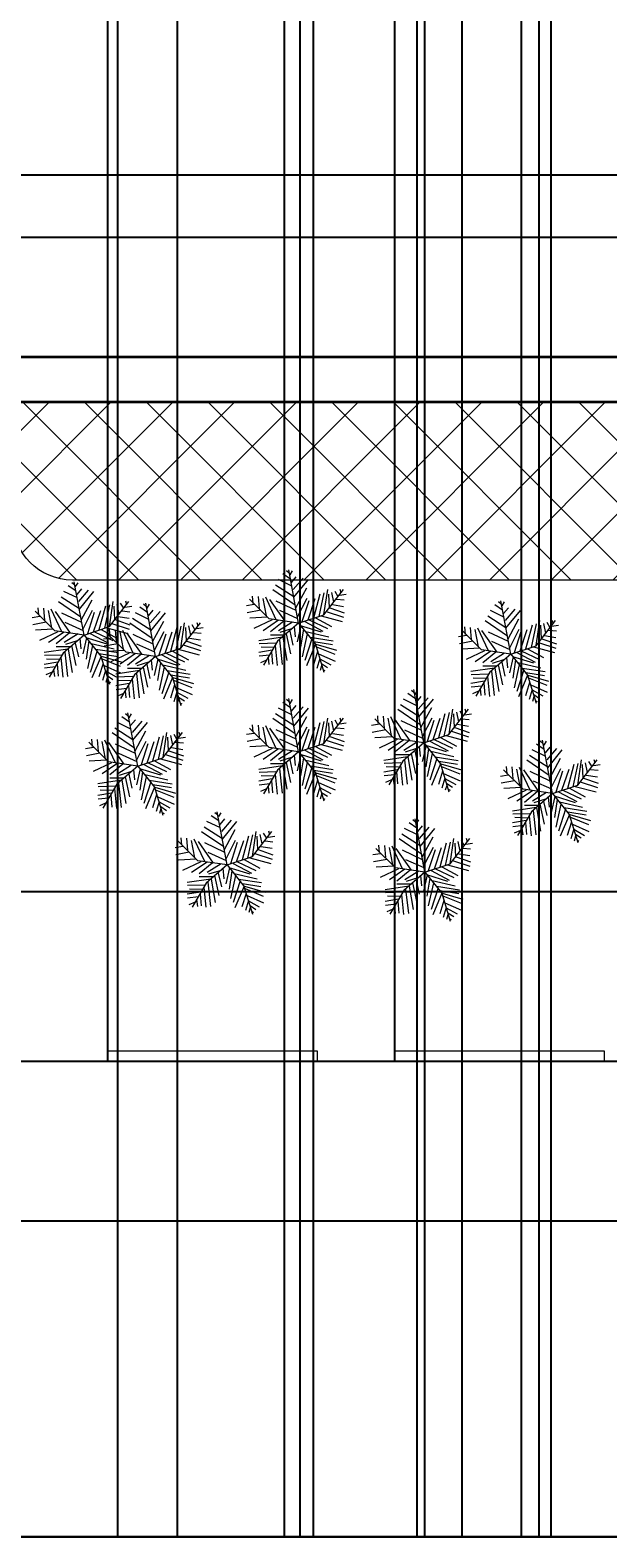
# Model space of a CAD drawing. Units: inches. Extents: x 818 to 1898, y 976 to 2364.
# Tile 16 of 96: x 1434 to 1550, y 976 to 1277. Entities that reach past the tile are written whole.
import ezdxf

# ---------------------------------------------------------------- set-up
doc = ezdxf.new("R2010")
doc.units = ezdxf.units.IN
doc.header["$LTSCALE"] = 5
doc.header["$MEASUREMENT"] = 0
for name, color, linetype, lineweight in [('A-ANNO-DIMS', 2, 'Continuous', 18), ('C-PAVE-PATT', 8, 'Continuous', 9), ('C-PROP', 7, 'Continuous', 35), ('C-ROAD', 8, 'Continuous', 25), ('C-ROAD-MRKG', 7, 'Continuous', 13), ('L-PAVE', 8, 'Continuous', 18)]:
    doc.layers.add(name, color=color, linetype=linetype, lineweight=lineweight)
doc.layers.add('L-PLNT', color=116, linetype='Continuous', lineweight=13, true_color=0x136734)
doc.styles.get("Standard").update_dxf_attribs({"font": 'arial.ttf'})
doc.dimstyles.get("Standard").update_dxf_attribs({"dimtxt": 0.18, "dimasz": 0.18, "dimexe": 0.18, "dimexo": 0.0625, "dimgap": 0.09, "dimtad": 0, "dimtih": 1, "dimtoh": 1, "dimdec": 4, "dimzin": 0, "dimdsep": 46, "dimtxsty": 'Standard', "dimcen": 0.09, "dimadec": 0, "dimazin": 0, "dimtfac": 1, "dimtdec": 4, "dimtofl": 0, "dimtmove": 0, "dimatfit": 3, "dimfxl": 1, "dimtolj": 1, "dimtzin": 0, "dimarcsym": 0})

# ---------------------------------------------------------------- blocks, each defined once
blk = doc.blocks.new('SHRUB-ACCENT')
for p, q in [((9.08, 17.24), (6.37, 18.54)), ((8.8, 18.63), (7.25, 19.67)), ((8.53, 19.84), (7.99, 20.28)), ((10.44, 9.82), (8.47, 20.47)), ((8.74, 19.5), (9.21, 20.28)), ((9.01, 17.93), (9.96, 19.06)), ((9.35, 16.54), (11.31, 18.8)), ((9.48, 14.98), (12.39, 18.54)), ((1.35, 13.77), (1.22, 15.24)), ((2.3, 15.16), (2.51, 12.72)), ((9.75, 13.42), (5.28, 16.46)), ((9.48, 15.07), (5.82, 17.41)), ((9.89, 12.9), (12.06, 16.89)), ((13.48, 10.9), (14.76, 15.68)), ((14.56, 11.16), (15.58, 15.85)), ((15.49, 11.5), (19.41, 16.55)), ((15.51, 11.51), (16.25, 16.54)), ((16.39, 15.59), (16.53, 12.9)), ((17, 15.94), (17.41, 14.03)), ((17.68, 16.2), (18.29, 15.16)), ((18.62, 15.42), (19.98, 15.59)), ((18.69, 16.63), (18.9, 15.94)), ((1.56, 13.51), (0, 13.25)), ((2.84, 12.38), (0.14, 11.86)), ((4.55, 10.66), (0.62, 14.58)), ((3.25, 14.72), (3.93, 11.25)), ((3.79, 15.07), (5.89, 10.55)), ((7.72, 10.21), (4.67, 14.55)), ((5.89, 14.29), (9.89, 12.38)), ((6.57, 12.38), (10.23, 10.73)), ((10.23, 11.07), (12.12, 14.81)), ((11.17, 10.12), (12.53, 14.37)), ((12.33, 10.47), (13.75, 14.72)), ((15.98, 12.12), (19.44, 10.99)), ((16.66, 12.9), (19.57, 11.86)), ((17.2, 13.51), (19.44, 13.16)), ((18.02, 14.63), (19.57, 14.46)), ((4.2, 10.99), (0.68, 10.81)), ((5.15, 10.47), (1.49, 8.73)), ((6.43, 10.38), (3.32, 8.3)), ((10.44, 9.82), (4.55, 10.66)), ((7.45, 10.21), (4.81, 8.04)), ((10.44, 9.82), (6.23, 6.17)), ((9.21, 10.03), (6.43, 8.3)), ((9.55, 9.16), (9.75, 7.08)), ((10.9, 9.25), (10.16, 6.04)), ((10.44, 9.82), (15.49, 11.5)), ((10.44, 9.82), (13.8, 5.61)), ((10.77, 9.34), (14.97, 8.04)), ((11.65, 10.12), (15.31, 8.21)), ((12.53, 10.47), (16.19, 8.73)), ((13.82, 10.9), (17, 9.16)), ((14.97, 11.25), (19.17, 10.12)), ((7.18, 6.99), (2.44, 6.3)), ((6.23, 6.17), (3.43, 1.4)), ((7.59, 7.43), (4.81, 7.43)), ((6.57, 6.39), (7.11, 1.52)), ((9.21, 8.73), (6.7, 7.95)), ((7.25, 6.99), (8.06, 2.31)), ((7.92, 7.69), (8.8, 3.69)), ((8.67, 8.21), (9.28, 5.43)), ((11.38, 8.64), (10.84, 5)), ((12.12, 7.69), (11.11, 3.09)), ((13.07, 6.65), (11.65, 2.31)), ((11.85, 8.12), (16.46, 7.08)), ((12.73, 6.99), (17.34, 6.3)), ((13.48, 6.13), (17.2, 5.52)), ((5.15, 4.39), (2.44, 3.95)), ((5.89, 5.78), (2.51, 5.69)), ((4.67, 3.43), (2.51, 3.17)), ((5.42, 4.91), (2.91, 5)), ((5.01, 4.04), (5.21, 1.61)), ((5.76, 5.34), (6.16, 1.35)), ((13.82, 5.6), (11.99, 1.26)), ((14.22, 4.13), (13.41, 1.44)), ((13.8, 5.61), (15.49, 0)), ((13.88, 5.6), (18.02, 4.39)), ((14.02, 5.08), (17.68, 3.61)), ((14.43, 3.69), (17.74, 2.22)), ((4, 2.39), (2.78, 1.87)), ((4.33, 2.91), (4.47, 1.52)), ((14.7, 2.74), (14.09, 0.74)), ((14.7, 2.65), (16.86, 1.44)), ((15.04, 1.26), (14.76, 0.31)), ((15.04, 1.7), (16.19, 0.92)), ((15.44, 0.48), (15.71, 0.31))]:
    blk.add_line(p, q)
blk = doc.blocks.new('LANE-STRIPE')
at = {"ltscale": 5}
for p, q in [((0, 2), (42, 2)), ((0, 2), (0, 0)), ((0, 0), (42, 0)), ((42, 2), (42, 0))]:
    blk.add_line(p, q, dxfattribs=at)
blk = doc.blocks.new('*D56')
at = {"layer": 'A-ANNO-DIMS', "color": 0, "lineweight": -2, "ltscale": 5, "transparency": 16777216}
for p, q in [((885.95, 1167.31), (885.95, 975.66)), ((1828.91, 1167.31), (1828.91, 975.66)), ((886.13, 975.84), (1357.14, 975.84)), ((1828.73, 975.84), (1357.72, 975.84))]:
    blk.add_line(p, q, dxfattribs=at)
at = {"layer": 'A-ANNO-DIMS', "color": 0, "ltscale": 5, "transparency": 16777216}
for points in [[(886.13, 975.87), (886.13, 975.81), (885.95, 975.84)], [(1828.73, 975.87), (1828.73, 975.81), (1828.91, 975.84)]]:
    blk.add_solid(points, dxfattribs=at)
at = {"layer": 'Defpoints', "color": 0, "ltscale": 5, "transparency": 16777216}
for p in [(885.95, 1167.37), (1828.91, 1167.37), (1828.91, 975.84)]:
    blk.add_point(p, dxfattribs=at)
at = {"layer": 'A-ANNO-DIMS', "color": 0, "ltscale": 5, "transparency": 16777216, "insert": (1357.43, 975.84), "char_height": 0.18, "attachment_point": 5}
blk.add_mtext('\\A1;943', dxfattribs=at)
blk = doc.blocks.new('*D58')
at = {"layer": 'A-ANNO-DIMS', "color": 0, "lineweight": -2, "ltscale": 5, "transparency": 16777216}
for p, q in [((881.51, 1159.31), (881.51, 975.66)), ((1834.44, 1145.13), (1834.44, 975.66)), ((881.69, 975.84), (1357.68, 975.84)), ((1834.26, 975.84), (1358.26, 975.84))]:
    blk.add_line(p, q, dxfattribs=at)
at = {"layer": 'A-ANNO-DIMS', "color": 0, "ltscale": 5, "transparency": 16777216}
for points in [[(881.69, 975.87), (881.69, 975.81), (881.51, 975.84)], [(1834.26, 975.87), (1834.26, 975.81), (1834.44, 975.84)]]:
    blk.add_solid(points, dxfattribs=at)
at = {"layer": 'Defpoints', "color": 0, "ltscale": 5, "transparency": 16777216}
for p in [(881.51, 1159.38), (1834.44, 1145.19), (1834.44, 975.84)]:
    blk.add_point(p, dxfattribs=at)
at = {"layer": 'A-ANNO-DIMS', "color": 0, "ltscale": 5, "transparency": 16777216, "insert": (1357.97, 975.84), "char_height": 0.18, "attachment_point": 5}
blk.add_mtext('\\A1;953', dxfattribs=at)
blk = doc.blocks.new('*D65')
at = {"layer": 'A-ANNO-DIMS', "color": 0, "lineweight": -2, "ltscale": 5, "transparency": 16777216}
for p, q in [((1430.73, 1346.02), (1430.73, 975.66)), ((1714.73, 1346.02), (1714.73, 975.66)), ((1430.91, 975.84), (1572.44, 975.84)), ((1714.55, 975.84), (1573.02, 975.84))]:
    blk.add_line(p, q, dxfattribs=at)
at = {"layer": 'A-ANNO-DIMS', "color": 0, "ltscale": 5, "transparency": 16777216}
for points in [[(1430.91, 975.87), (1430.91, 975.81), (1430.73, 975.84)], [(1714.55, 975.87), (1714.55, 975.81), (1714.73, 975.84)]]:
    blk.add_solid(points, dxfattribs=at)
at = {"layer": 'Defpoints', "color": 0, "ltscale": 5, "transparency": 16777216}
for p in [(1430.73, 1346.08), (1714.73, 1346.08), (1714.73, 975.84)]:
    blk.add_point(p, dxfattribs=at)
at = {"layer": 'A-ANNO-DIMS', "color": 0, "ltscale": 5, "transparency": 16777216, "insert": (1572.73, 975.84), "char_height": 0.18, "attachment_point": 5}
blk.add_mtext('\\A1;284', dxfattribs=at)
blk = doc.blocks.new('*D89')
at = {"layer": 'A-ANNO-DIMS', "color": 0, "lineweight": -2, "ltscale": 5, "transparency": 16777216}
for p, q in [((905.01, 1071.06), (1897.92, 1071.06)), ((1897.74, 1070.88), (1897.74, 1055.28)), ((1897.74, 1039.32), (1897.74, 1054.92)), ((896.18, 1039.14), (1897.92, 1039.14))]:
    blk.add_line(p, q, dxfattribs=at)
at = {"layer": 'A-ANNO-DIMS', "color": 0, "ltscale": 5, "transparency": 16777216}
for points in [[(1897.71, 1070.88), (1897.77, 1070.88), (1897.74, 1071.06)], [(1897.71, 1039.32), (1897.77, 1039.32), (1897.74, 1039.14)]]:
    blk.add_solid(points, dxfattribs=at)
at = {"layer": 'Defpoints', "color": 0, "ltscale": 5, "transparency": 16777216}
for p in [(904.95, 1071.06), (1897.74, 1071.06), (896.11, 1039.14)]:
    blk.add_point(p, dxfattribs=at)
at = {"layer": 'A-ANNO-DIMS', "color": 0, "ltscale": 5, "transparency": 16777216, "insert": (1897.74, 1055.1), "char_height": 0.18, "attachment_point": 5}
blk.add_mtext('\\A1;31.91', dxfattribs=at)
blk = doc.blocks.new('*D99')
at = {"layer": 'A-ANNO-DIMS', "color": 0, "lineweight": -2, "ltscale": 5, "transparency": 16777216}
for p, q in [((1391.88, 1071.12), (1391.88, 2363.87)), ((1392.06, 2363.69), (1420.45, 2363.69)), ((1449.64, 2363.69), (1421.24, 2363.69)), ((1449.82, 1071.12), (1449.82, 2363.87))]:
    blk.add_line(p, q, dxfattribs=at)
at = {"layer": 'A-ANNO-DIMS', "color": 0, "ltscale": 5, "transparency": 16777216}
for points in [[(1392.06, 2363.72), (1392.06, 2363.66), (1391.88, 2363.69)], [(1449.64, 2363.72), (1449.64, 2363.66), (1449.82, 2363.69)]]:
    blk.add_solid(points, dxfattribs=at)
at = {"layer": 'Defpoints', "color": 0, "ltscale": 5, "transparency": 16777216}
for p in [(1449.82, 2363.69), (1391.88, 1071.06), (1449.82, 1071.06)]:
    blk.add_point(p, dxfattribs=at)
at = {"layer": 'A-ANNO-DIMS', "color": 0, "ltscale": 5, "transparency": 16777216, "insert": (1420.85, 2363.69), "char_height": 0.18, "attachment_point": 5}
blk.add_mtext('\\A1;57.94', dxfattribs=at)
blk = doc.blocks.new('*D100')
at = {"layer": 'A-ANNO-DIMS', "color": 0, "lineweight": -2, "ltscale": 5, "transparency": 16777216}
for p, q in [((1449.82, 1071.12), (1449.82, 2363.87)), ((1450, 2363.69), (1478.17, 2363.69)), ((1507.12, 2363.69), (1478.95, 2363.69)), ((1507.3, 1071.12), (1507.3, 2363.87))]:
    blk.add_line(p, q, dxfattribs=at)
at = {"layer": 'A-ANNO-DIMS', "color": 0, "ltscale": 5, "transparency": 16777216}
for points in [[(1450, 2363.72), (1450, 2363.66), (1449.82, 2363.69)], [(1507.12, 2363.72), (1507.12, 2363.66), (1507.3, 2363.69)]]:
    blk.add_solid(points, dxfattribs=at)
at = {"layer": 'Defpoints', "color": 0, "ltscale": 5, "transparency": 16777216}
for p in [(1507.3, 2363.69), (1449.82, 1071.06), (1507.3, 1071.06)]:
    blk.add_point(p, dxfattribs=at)
at = {"layer": 'A-ANNO-DIMS', "color": 0, "ltscale": 5, "transparency": 16777216, "insert": (1478.56, 2363.69), "char_height": 0.18, "attachment_point": 5}
blk.add_mtext('\\A1;57.48', dxfattribs=at)
blk = doc.blocks.new('*D101')
at = {"layer": 'A-ANNO-DIMS', "color": 0, "lineweight": -2, "ltscale": 5, "transparency": 16777216}
for p, q in [((1507.3, 1071.12), (1507.3, 2363.87)), ((1507.48, 2363.69), (1536, 2363.69)), ((1565.3, 2363.69), (1536.78, 2363.69)), ((1565.48, 1071.12), (1565.48, 2363.87))]:
    blk.add_line(p, q, dxfattribs=at)
at = {"layer": 'A-ANNO-DIMS', "color": 0, "ltscale": 5, "transparency": 16777216}
for points in [[(1507.48, 2363.72), (1507.48, 2363.66), (1507.3, 2363.69)], [(1565.3, 2363.72), (1565.3, 2363.66), (1565.48, 2363.69)]]:
    blk.add_solid(points, dxfattribs=at)
at = {"layer": 'Defpoints', "color": 0, "ltscale": 5, "transparency": 16777216}
for p in [(1565.48, 2363.69), (1507.3, 1071.06), (1565.48, 1071.06)]:
    blk.add_point(p, dxfattribs=at)
at = {"layer": 'A-ANNO-DIMS', "color": 0, "ltscale": 5, "transparency": 16777216, "insert": (1536.39, 2363.69), "char_height": 0.18, "attachment_point": 5}
blk.add_mtext('\\A1;58.19', dxfattribs=at)
blk = doc.blocks.new('*D110')
at = {"layer": 'A-ANNO-DIMS', "color": 0, "lineweight": -2, "ltscale": 5, "transparency": 16777216}
for p, q in [((1164.62, 1248.46), (1897.92, 1248.46)), ((1897.74, 1248.28), (1897.74, 1242.4)), ((1897.74, 1236.14), (1897.74, 1242.03)), ((1116.25, 1235.96), (1897.92, 1235.96))]:
    blk.add_line(p, q, dxfattribs=at)
at = {"layer": 'A-ANNO-DIMS', "color": 0, "ltscale": 5, "transparency": 16777216}
for points in [[(1897.71, 1248.28), (1897.77, 1248.28), (1897.74, 1248.46)], [(1897.71, 1236.14), (1897.77, 1236.14), (1897.74, 1235.96)]]:
    blk.add_solid(points, dxfattribs=at)
at = {"layer": 'Defpoints', "color": 0, "ltscale": 5, "transparency": 16777216}
for p in [(1164.56, 1248.46), (1116.19, 1235.96), (1897.74, 1235.96)]:
    blk.add_point(p, dxfattribs=at)
at = {"layer": 'A-ANNO-DIMS', "color": 0, "ltscale": 5, "transparency": 16777216, "insert": (1897.74, 1242.21), "char_height": 0.18, "attachment_point": 5}
blk.add_mtext('\\A1;12.498', dxfattribs=at)
blk = doc.blocks.new('*D159')
at = {"layer": 'A-ANNO-DIMS', "color": 0, "lineweight": -2, "ltscale": 5, "transparency": 16777216}
for p, q in [((1206.73, 1687.02), (1206.73, 975.66)), ((1463.73, 1687.02), (1463.73, 975.66)), ((1206.91, 975.84), (1334.93, 975.84)), ((1463.55, 975.84), (1335.52, 975.84))]:
    blk.add_line(p, q, dxfattribs=at)
at = {"layer": 'A-ANNO-DIMS', "color": 0, "ltscale": 5, "transparency": 16777216}
for points in [[(1206.91, 975.87), (1206.91, 975.81), (1206.73, 975.84)], [(1463.55, 975.87), (1463.55, 975.81), (1463.73, 975.84)]]:
    blk.add_solid(points, dxfattribs=at)
at = {"layer": 'Defpoints', "color": 0, "ltscale": 5, "transparency": 16777216}
for p in [(1206.73, 1687.08), (1463.73, 1687.08), (1463.73, 975.84)]:
    blk.add_point(p, dxfattribs=at)
at = {"layer": 'A-ANNO-DIMS', "color": 0, "ltscale": 5, "transparency": 16777216, "insert": (1335.23, 975.84), "char_height": 0.18, "attachment_point": 5}
blk.add_mtext('\\A1;257', dxfattribs=at)
blk = doc.blocks.new('*D160')
at = {"layer": 'A-ANNO-DIMS', "color": 0, "lineweight": -2, "ltscale": 5, "transparency": 16777216}
for p, q in [((1463.73, 1687.02), (1463.73, 975.66)), ((1511.73, 1687.02), (1511.73, 975.66)), ((1463.91, 975.84), (1487.5, 975.84)), ((1511.55, 975.84), (1487.95, 975.84))]:
    blk.add_line(p, q, dxfattribs=at)
at = {"layer": 'A-ANNO-DIMS', "color": 0, "ltscale": 5, "transparency": 16777216}
for points in [[(1463.91, 975.87), (1463.91, 975.81), (1463.73, 975.84)], [(1511.55, 975.87), (1511.55, 975.81), (1511.73, 975.84)]]:
    blk.add_solid(points, dxfattribs=at)
at = {"layer": 'Defpoints', "color": 0, "ltscale": 5, "transparency": 16777216}
for p in [(1463.73, 1687.08), (1511.73, 1687.08), (1511.73, 975.84)]:
    blk.add_point(p, dxfattribs=at)
at = {"layer": 'A-ANNO-DIMS', "color": 0, "ltscale": 5, "transparency": 16777216, "insert": (1487.73, 975.84), "char_height": 0.18, "attachment_point": 5}
blk.add_mtext('\\A1;48', dxfattribs=at)
blk = doc.blocks.new('*D182')
at = {"layer": 'A-ANNO-DIMS', "color": 0, "lineweight": -2, "ltscale": 5, "transparency": 16777216}
for p, q in [((1463.73, 1687.02), (1463.73, 975.66)), ((1559.73, 1687.02), (1559.73, 975.66)), ((1463.91, 975.84), (1511.51, 975.84)), ((1559.55, 975.84), (1511.94, 975.84))]:
    blk.add_line(p, q, dxfattribs=at)
at = {"layer": 'A-ANNO-DIMS', "color": 0, "ltscale": 5, "transparency": 16777216}
for points in [[(1463.91, 975.87), (1463.91, 975.81), (1463.73, 975.84)], [(1559.55, 975.87), (1559.55, 975.81), (1559.73, 975.84)]]:
    blk.add_solid(points, dxfattribs=at)
at = {"layer": 'Defpoints', "color": 0, "ltscale": 5, "transparency": 16777216}
for p in [(1463.73, 1687.08), (1559.73, 1687.08), (1559.73, 975.84)]:
    blk.add_point(p, dxfattribs=at)
at = {"layer": 'A-ANNO-DIMS', "color": 0, "ltscale": 5, "transparency": 16777216, "insert": (1511.73, 975.84), "char_height": 0.18, "attachment_point": 5}
blk.add_mtext('\\A1;96', dxfattribs=at)
blk = doc.blocks.new('*D189')
at = {"layer": 'A-ANNO-DIMS', "color": 0, "lineweight": -2, "ltscale": 5, "transparency": 16777216}
for p, q in [((1430.73, 1346.02), (1430.73, 975.66)), ((1490.92, 1346.02), (1490.92, 975.66)), ((1430.91, 975.84), (1460.43, 975.84)), ((1490.74, 975.84), (1461.22, 975.84))]:
    blk.add_line(p, q, dxfattribs=at)
at = {"layer": 'A-ANNO-DIMS', "color": 0, "ltscale": 5, "transparency": 16777216}
for points in [[(1430.91, 975.87), (1430.91, 975.81), (1430.73, 975.84)], [(1490.74, 975.87), (1490.74, 975.81), (1490.92, 975.84)]]:
    blk.add_solid(points, dxfattribs=at)
at = {"layer": 'Defpoints', "color": 0, "ltscale": 5, "transparency": 16777216}
for p in [(1430.73, 1346.08), (1490.92, 1346.08), (1490.92, 975.84)]:
    blk.add_point(p, dxfattribs=at)
at = {"layer": 'A-ANNO-DIMS', "color": 0, "ltscale": 5, "transparency": 16777216, "insert": (1460.82, 975.84), "char_height": 0.18, "attachment_point": 5}
blk.add_mtext('\\A1;60.19', dxfattribs=at)
blk = doc.blocks.new('*D198')
at = {"layer": 'A-ANNO-DIMS', "color": 0, "lineweight": -2, "ltscale": 5, "transparency": 16777216}
for p, q in [((1741.84, 1545.02), (1741.84, 975.66)), ((1430.73, 1346.02), (1430.73, 975.66)), ((1430.91, 975.84), (1585.91, 975.84)), ((1741.66, 975.84), (1586.66, 975.84))]:
    blk.add_line(p, q, dxfattribs=at)
at = {"layer": 'A-ANNO-DIMS', "color": 0, "ltscale": 5, "transparency": 16777216}
for points in [[(1430.91, 975.87), (1430.91, 975.81), (1430.73, 975.84)], [(1741.66, 975.87), (1741.66, 975.81), (1741.84, 975.84)]]:
    blk.add_solid(points, dxfattribs=at)
at = {"layer": 'Defpoints', "color": 0, "ltscale": 5, "transparency": 16777216}
for p in [(1741.84, 1545.08), (1430.73, 1346.08), (1741.84, 975.84)]:
    blk.add_point(p, dxfattribs=at)
at = {"layer": 'A-ANNO-DIMS', "color": 0, "ltscale": 5, "transparency": 16777216, "insert": (1586.28, 975.84), "char_height": 0.18, "attachment_point": 5}
blk.add_mtext('\\A1;311.1', dxfattribs=at)
blk = doc.blocks.new('*D214')
at = {"layer": 'A-ANNO-DIMS', "color": 0, "lineweight": -2, "ltscale": 5, "transparency": 16777216}
for p, q in [((1511.73, 1687.02), (1511.73, 975.66)), ((1714.73, 1687.02), (1714.73, 975.66)), ((1511.91, 975.84), (1612.93, 975.84)), ((1714.55, 975.84), (1613.52, 975.84))]:
    blk.add_line(p, q, dxfattribs=at)
at = {"layer": 'A-ANNO-DIMS', "color": 0, "ltscale": 5, "transparency": 16777216}
for points in [[(1511.91, 975.87), (1511.91, 975.81), (1511.73, 975.84)], [(1714.55, 975.87), (1714.55, 975.81), (1714.73, 975.84)]]:
    blk.add_solid(points, dxfattribs=at)
at = {"layer": 'Defpoints', "color": 0, "ltscale": 5, "transparency": 16777216}
for p in [(1511.73, 1687.08), (1714.73, 1687.08), (1714.73, 975.84)]:
    blk.add_point(p, dxfattribs=at)
at = {"layer": 'A-ANNO-DIMS', "color": 0, "ltscale": 5, "transparency": 16777216, "insert": (1613.23, 975.84), "char_height": 0.18, "attachment_point": 5}
blk.add_mtext('\\A1;203', dxfattribs=at)
blk = doc.blocks.new('*D224')
at = {"layer": 'A-ANNO-DIMS', "color": 0, "lineweight": -2, "ltscale": 5, "transparency": 16777216}
for p, q in [((1520.73, 1837.52), (1520.73, 975.66)), ((1532.59, 1837.52), (1532.59, 975.66)), ((1520.91, 975.84), (1526.2, 975.84)), ((1532.41, 975.84), (1527.11, 975.84))]:
    blk.add_line(p, q, dxfattribs=at)
at = {"layer": 'A-ANNO-DIMS', "color": 0, "ltscale": 5, "transparency": 16777216}
for points in [[(1520.91, 975.87), (1520.91, 975.81), (1520.73, 975.84)], [(1532.41, 975.87), (1532.41, 975.81), (1532.59, 975.84)]]:
    blk.add_solid(points, dxfattribs=at)
at = {"layer": 'Defpoints', "color": 0, "ltscale": 5, "transparency": 16777216}
for p in [(1520.73, 1837.58), (1532.59, 1837.58), (1532.59, 975.84)]:
    blk.add_point(p, dxfattribs=at)
at = {"layer": 'A-ANNO-DIMS', "color": 0, "ltscale": 5, "transparency": 16777216, "insert": (1526.66, 975.84), "char_height": 0.18, "attachment_point": 5}
blk.add_mtext('\\A1;11.868', dxfattribs=at)
blk = doc.blocks.new('*D226')
at = {"layer": 'A-ANNO-DIMS', "color": 0, "lineweight": -2, "ltscale": 5, "transparency": 16777216}
for p, q in [((1536.17, 1774.47), (1536.17, 975.66)), ((1520.73, 1773.02), (1520.73, 975.66)), ((1520.91, 975.84), (1527.99, 975.84)), ((1535.99, 975.84), (1528.9, 975.84))]:
    blk.add_line(p, q, dxfattribs=at)
at = {"layer": 'A-ANNO-DIMS', "color": 0, "ltscale": 5, "transparency": 16777216}
for points in [[(1520.91, 975.87), (1520.91, 975.81), (1520.73, 975.84)], [(1535.99, 975.87), (1535.99, 975.81), (1536.17, 975.84)]]:
    blk.add_solid(points, dxfattribs=at)
at = {"layer": 'Defpoints', "color": 0, "ltscale": 5, "transparency": 16777216}
for p in [(1536.17, 1774.53), (1520.73, 1773.08), (1536.17, 975.84)]:
    blk.add_point(p, dxfattribs=at)
at = {"layer": 'A-ANNO-DIMS', "color": 0, "ltscale": 5, "transparency": 16777216, "insert": (1528.45, 975.84), "char_height": 0.18, "attachment_point": 5}
blk.add_mtext('\\A1;15.445', dxfattribs=at)
blk = doc.blocks.new('*D242')
at = {"layer": 'A-ANNO-DIMS', "color": 0, "lineweight": -2, "ltscale": 5, "transparency": 16777216}
for p, q in [((1488.26, 1948.6), (1488.26, 975.66)), ((1513.23, 1948.6), (1513.23, 975.66)), ((1488.44, 975.84), (1500.35, 975.84)), ((1513.05, 975.84), (1501.14, 975.84))]:
    blk.add_line(p, q, dxfattribs=at)
at = {"layer": 'A-ANNO-DIMS', "color": 0, "ltscale": 5, "transparency": 16777216}
for points in [[(1488.44, 975.87), (1488.44, 975.81), (1488.26, 975.84)], [(1513.05, 975.87), (1513.05, 975.81), (1513.23, 975.84)]]:
    blk.add_solid(points, dxfattribs=at)
at = {"layer": 'Defpoints', "color": 0, "ltscale": 5, "transparency": 16777216}
for p in [(1488.26, 1948.66), (1513.23, 1948.66), (1513.23, 975.84)]:
    blk.add_point(p, dxfattribs=at)
at = {"layer": 'A-ANNO-DIMS', "color": 0, "ltscale": 5, "transparency": 16777216, "insert": (1500.74, 975.84), "char_height": 0.18, "attachment_point": 5}
blk.add_mtext('\\A1;24.97', dxfattribs=at)
blk = doc.blocks.new('*D243')
at = {"layer": 'A-ANNO-DIMS', "color": 0, "lineweight": -2, "ltscale": 5, "transparency": 16777216}
for p, q in [((1451.77, 2020.02), (1451.77, 975.66)), ((1590.73, 2020.02), (1590.73, 975.66)), ((1451.95, 975.84), (1520.79, 975.84)), ((1590.55, 975.84), (1521.7, 975.84))]:
    blk.add_line(p, q, dxfattribs=at)
at = {"layer": 'A-ANNO-DIMS', "color": 0, "ltscale": 5, "transparency": 16777216}
for points in [[(1451.95, 975.87), (1451.95, 975.81), (1451.77, 975.84)], [(1590.55, 975.87), (1590.55, 975.81), (1590.73, 975.84)]]:
    blk.add_solid(points, dxfattribs=at)
at = {"layer": 'Defpoints', "color": 0, "ltscale": 5, "transparency": 16777216}
for p in [(1451.77, 2020.08), (1590.73, 2020.08), (1590.73, 975.84)]:
    blk.add_point(p, dxfattribs=at)
at = {"layer": 'A-ANNO-DIMS', "color": 0, "ltscale": 5, "transparency": 16777216, "insert": (1521.25, 975.84), "char_height": 0.18, "attachment_point": 5}
blk.add_mtext('\\A1;138.96', dxfattribs=at)
blk = doc.blocks.new('*D253')
at = {"layer": 'A-ANNO-DIMS', "color": 0, "lineweight": -2, "ltscale": 5, "transparency": 16777216}
for p, q in [((1485.12, 2053.02), (1485.12, 975.66)), ((1538.52, 2053.02), (1538.52, 975.66)), ((1485.3, 975.84), (1511.42, 975.84)), ((1538.34, 975.84), (1512.21, 975.84))]:
    blk.add_line(p, q, dxfattribs=at)
at = {"layer": 'A-ANNO-DIMS', "color": 0, "ltscale": 5, "transparency": 16777216}
for points in [[(1485.3, 975.87), (1485.3, 975.81), (1485.12, 975.84)], [(1538.34, 975.87), (1538.34, 975.81), (1538.52, 975.84)]]:
    blk.add_solid(points, dxfattribs=at)
at = {"layer": 'Defpoints', "color": 0, "ltscale": 5, "transparency": 16777216}
for p in [(1485.12, 2053.08), (1538.52, 2053.08), (1538.52, 975.84)]:
    blk.add_point(p, dxfattribs=at)
at = {"layer": 'A-ANNO-DIMS', "color": 0, "ltscale": 5, "transparency": 16777216, "insert": (1511.82, 975.84), "char_height": 0.18, "attachment_point": 5}
blk.add_mtext('\\A1;53.39', dxfattribs=at)

msp = doc.modelspace()

# ---------------------------------------------------------------- hatches: boundary and pattern name
at = {"layer": 'C-PAVE-PATT', "ltscale": 5}
h = msp.add_hatch(dxfattribs=at)
h.set_pattern_fill('ANSI37', color=256, scale=70)
h.paths.add_polyline_path([(1071.7252, 1202.9642), (885.9457, 1202.9642), (885.9457, 1167.3717), (1059.7252, 1167.3717, 0.41421356), (1071.7252, 1179.3717)])
h.paths.add_polyline_path([(1828.9123, 1202.9642), (1430.7251, 1202.9642), (1430.7251, 1179.3717, 0.41421356), (1442.7252, 1167.3717), (1828.9123, 1167.3717)])

# ---------------------------------------------------------------- linework, layer by layer
at = {"layer": 'C-PROP', "ltscale": 5}
for p, q in [((1789.7173, 1211.9642), (1430.7251, 1211.9642)), ((1798.7173, 1202.9642), (992.7252, 1202.9642))]:
    msp.add_line(p, q, dxfattribs=at)
at = {"layer": 'C-ROAD', "ltscale": 5}
msp.add_lwpolyline([(1828.9123, 1104.9672), (896.1138, 1104.9672), (896.1138, 1039.1433), (1828.9123, 1039.1433)], close=True, dxfattribs=at)
at = {"layer": 'L-PAVE', "ltscale": 5}
msp.add_lwpolyline([(1430.7251, 1202.9642), (1828.9123, 1202.9642), (1828.9123, 1167.3717), (1442.7252, 1167.3717, -0.41421356), (1430.7251, 1179.3717)], format="xyb", close=True, dxfattribs=at)

# ---------------------------------------------------------------- block references
at = {"layer": 'C-ROAD-MRKG', "rotation": 180}
for p in [(1491.8208, 1073.0554), (1549.2994, 1073.0554)]:
    msp.add_blockref('LANE-STRIPE', p, dxfattribs=at)
at = {"layer": 'L-PLNT'}
for p in [(1477.5985, 1148.9297), (1434.6356, 1146.5448), (1448.9566, 1142.252), (1520.0841, 1142.729), (1502.6433, 1124.9779), (1445.3763, 1120.3112), (1477.5985, 1123.173), (1528.438, 1114.8259), (1463.2776, 1100.5167), (1502.8989, 1099.0858)]:
    msp.add_blockref('SHRUB-ACCENT', p, dxfattribs=at)

# ---------------------------------------------------------------- dimensions: what is measured, and where the dimension line sits
at = {"layer": 'A-ANNO-DIMS', "ltscale": 5}
for base, p1, p2, override, picture, middle in [((1449.8196, 2363.6929), (1391.8757, 1071.0552), (1449.8196, 1071.0552), {"dimdec": 2, "dimlfac": 1, "dimrnd": 0, "dimzin": 0, "dimdsep": 46, "dimlunit": 2}, '*D99', (1420.8477, 2363.6929)), ((1507.2982, 2363.6929), (1449.8196, 1071.0552), (1507.2982, 1071.0552), {"dimdec": 2, "dimlfac": 1, "dimrnd": 0, "dimzin": 0, "dimdsep": 46, "dimlunit": 2}, '*D100', (1478.5589, 2363.6929)), ((1565.4835, 2363.6929), (1507.2982, 1071.0552), (1565.4835, 1071.0552), {"dimdec": 2, "dimlfac": 1, "dimrnd": 0, "dimzin": 0, "dimdsep": 46, "dimlunit": 2}, '*D101', (1536.3908, 2363.6929)), ((1538.5155, 975.8433), (1485.1216, 2053.0782), (1538.5155, 2053.0782), {"dimdec": 2, "dimlfac": 1, "dimrnd": 0, "dimzin": 0, "dimdsep": 46, "dimlunit": 2}, '*D253', (1511.8185, 975.8433)), ((1590.7251, 975.8433), (1451.7698, 2020.0782), (1590.7251, 2020.0782), {"dimdec": 2, "dimlfac": 1, "dimrnd": 0, "dimzin": 0, "dimdsep": 46, "dimlunit": 2}, '*D243', (1521.2475, 975.8433)), ((1513.2306, 975.8433), (1488.2586, 1948.6602), (1513.2306, 1948.6602), {"dimdec": 2, "dimlfac": 1, "dimrnd": 0, "dimzin": 0, "dimdsep": 46, "dimlunit": 2}, '*D242', (1500.7446, 975.8433)), ((1532.593, 975.8433), (1520.7251, 1837.5823), (1532.593, 1837.5823), {"dimdec": 3, "dimlfac": 1, "dimrnd": 0, "dimzin": 0, "dimdsep": 46, "dimlunit": 2}, '*D224', (1526.6591, 975.8433)), ((1536.1698, 975.8433), (1520.7251, 1773.0782), (1536.1698, 1774.5283), {"dimdec": 3, "dimlfac": 1, "dimrnd": 0, "dimzin": 0, "dimdsep": 46, "dimlunit": 2}, '*D226', (1528.4475, 975.8433)), ((1463.7251, 975.8433), (1206.7251, 1687.0782), (1463.7251, 1687.0782), {"dimdec": 0, "dimlfac": 1, "dimrnd": 0, "dimzin": 0, "dimdsep": 46, "dimlunit": 2}, '*D159', (1335.2251, 975.8433)), ((1511.7251, 975.8433), (1463.7251, 1687.0782), (1511.7251, 1687.0782), {"dimdec": 0, "dimlfac": 1, "dimrnd": 0, "dimzin": 0, "dimdsep": 46, "dimlunit": 2}, '*D160', (1487.7251, 975.8433)), ((1559.7251, 975.8433), (1463.7251, 1687.0782), (1559.7251, 1687.0782), {"dimdec": 0, "dimlfac": 1, "dimrnd": 0, "dimzin": 0, "dimdsep": 46, "dimlunit": 2}, '*D182', (1511.7251, 975.8433)), ((1714.7251, 975.8433), (1511.7251, 1687.0782), (1714.7251, 1687.0782), {"dimdec": 0, "dimlfac": 1, "dimrnd": 0, "dimzin": 0, "dimdsep": 46, "dimlunit": 2}, '*D214', (1613.2251, 975.8433)), ((1741.8409, 975.8433), (1430.7251, 1346.0782), (1741.8409, 1545.0782), {"dimdec": 1, "dimlfac": 1, "dimrnd": 0, "dimzin": 0, "dimdsep": 46, "dimlunit": 2}, '*D198', (1586.283, 975.8433)), ((1714.7251, 975.8433), (1430.7251, 1346.0782), (1714.7251, 1346.0782), {"dimdec": 0, "dimlfac": 1, "dimrnd": 0, "dimzin": 0, "dimdsep": 46, "dimlunit": 2}, '*D65', (1572.7251, 975.8433)), ((1490.9163, 975.8433), (1430.7251, 1346.0782), (1490.9163, 1346.0782), {"dimdec": 2, "dimlfac": 1, "dimrnd": 0, "dimzin": 0, "dimdsep": 46, "dimlunit": 2}, '*D189', (1460.8207, 975.8433)), ((1828.9123, 975.8433), (885.9457, 1167.3717), (1828.9123, 1167.3717), {"dimdec": 0, "dimlfac": 1, "dimrnd": 0, "dimzin": 0, "dimdsep": 46, "dimlunit": 2}, '*D56', (1357.429, 975.8433)), ((1834.436, 975.8433), (881.5059, 1159.375), (1834.436, 1145.1942), {"dimdec": 0, "dimlfac": 1, "dimrnd": 0, "dimzin": 0, "dimdsep": 46, "dimlunit": 2}, '*D58', (1357.971, 975.8433))]:
    dim = msp.add_linear_dim(base=base, p1=p1, p2=p2, dimstyle='Standard', override=override, dxfattribs=at)
    dim.commit()
    dim.dimension.update_dxf_attribs({"geometry": picture, "text_midpoint": middle})
for base, p1, p2, override, picture, middle in [((1897.736, 1235.9642), (1164.5571, 1248.4622), (1116.1882, 1235.9642), {"dimdec": 3, "dimlfac": 1, "dimrnd": 0, "dimzin": 0, "dimdsep": 46, "dimlunit": 2}, '*D110', (1897.736, 1242.2132)), ((1897.736, 1071.0552), (896.1138, 1039.1433), (904.9504, 1071.0552), {"dimdec": 2, "dimlfac": 1, "dimrnd": 0, "dimzin": 0, "dimdsep": 46, "dimlunit": 2}, '*D89', (1897.736, 1055.0992))]:
    dim = msp.add_linear_dim(base=base, p1=p1, p2=p2, angle=90, dimstyle='Standard', override=override, dxfattribs=at)
    dim.commit()
    dim.dimension.update_dxf_attribs({"geometry": picture, "text_midpoint": middle})

doc.saveas('drawing.dxf')
